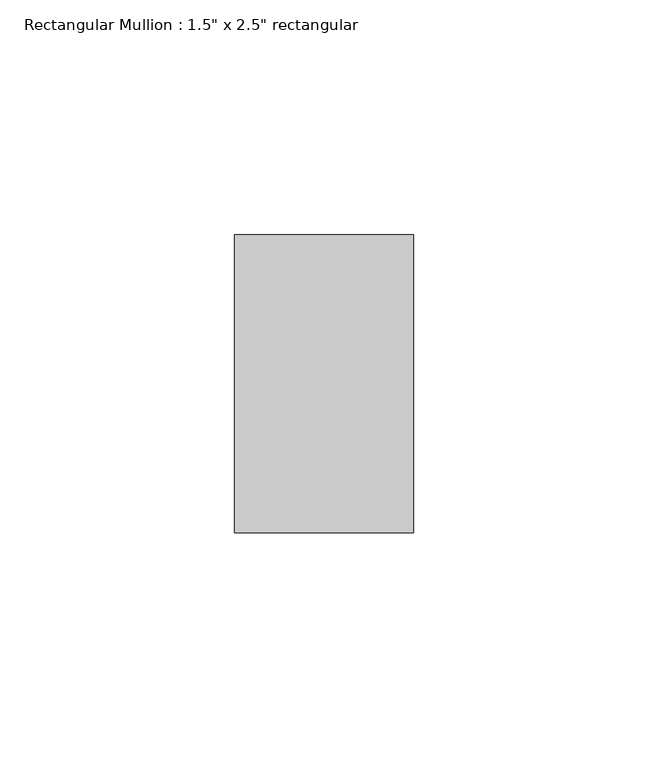
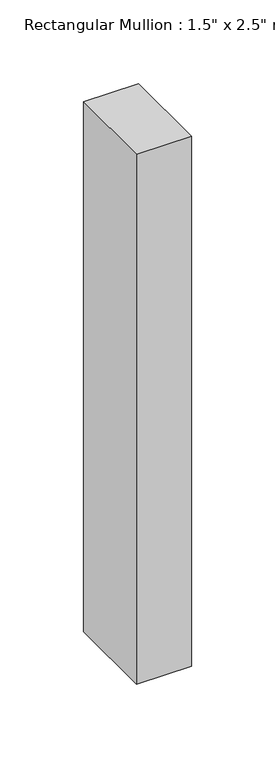
"""IFC4 building model written with IfcOpenShell, lengths in millimetres: member geometry."""

from ifc_helpers import new_model, si_unit, frame, origin, place, context, project, spatial, polyline, outline, extrude, source, transform, mapped, element, save


def member_18929904(model_context):
    return source(origin(), model_context, "Body", "SweptSolid", [
        extrude(outline(polyline([(0.0, 31.75), (0.0, -31.75), (-38.1, -31.75), (-38.1, 31.75), (0.0, 31.75)])), frame((0.0, 0.0, -387.35), z_axis=(0.0, 0.0, 1.0), x_axis=(1.0, 0.0, 0.0)), (0.0, 0.0, 1.0), 387.35),
    ])


if __name__ == "__main__":
    model = new_model("IFC4")
    model_context = context("Model", 3, world=origin())
    ifc_project = project(units=[si_unit("LENGTHUNIT", "METRE", prefix="MILLI")], contexts=[model_context])
    site = spatial("IfcSite", under=ifc_project)
    building = spatial("IfcBuilding", under=site)
    placement = place(None, origin())
    member_shape = member_18929904(model_context)
    element("IfcMember", 1, ObjectType="Rectangular Mullion : 1.5\" x 2.5\" rectangular", at=placement, inside=building, context=model_context, shape_type="MappedRepresentation", body=[
        mapped(member_shape, transform((0.0, 0.0, 0.0), x_axis=(1.0, 0.0, 0.0), y_axis=(0.0, 1.0, 0.0), z_axis=(0.0, 0.0, 1.0))),
    ])
    save(model, "model.ifc")

# Revit data of these elements
# Type "Rectangular Mullion : 1.5\" x 2.5\" rectangular"
#   built-in parameter 1007304 = 0.208333 (stored number, unit not read)
#   built-in parameter 1007301 = 0.0625 (stored number, unit not read)
#   built-in parameter 1007300 = 0.0625 (stored number, unit not read)
# Element 1 (IfcMember, "Rectangular Mullion : 1.5\" x 2.5\" rectangular")
#   Materials on its faces: "Aluminum"
# Materials
#   "Aluminum": class "Metal", colour RGB 247 247 247, transparency 0, Description = "Aluminum 6061", Cost = 0
